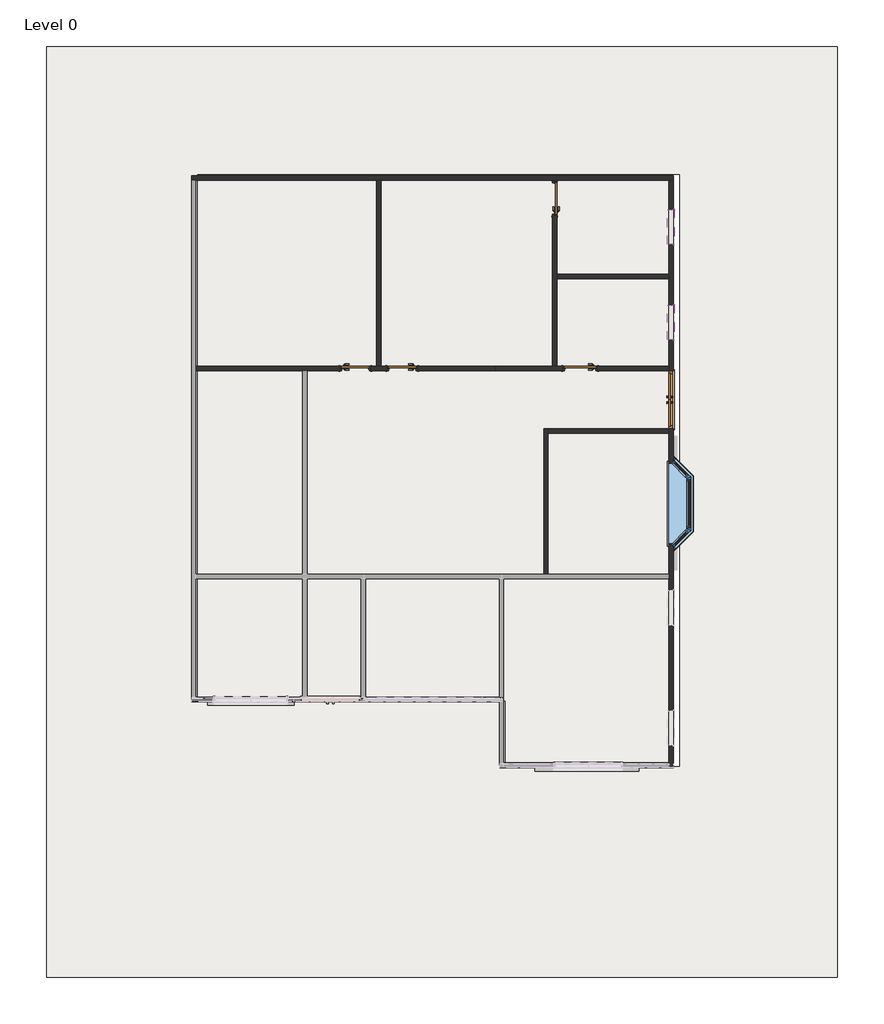
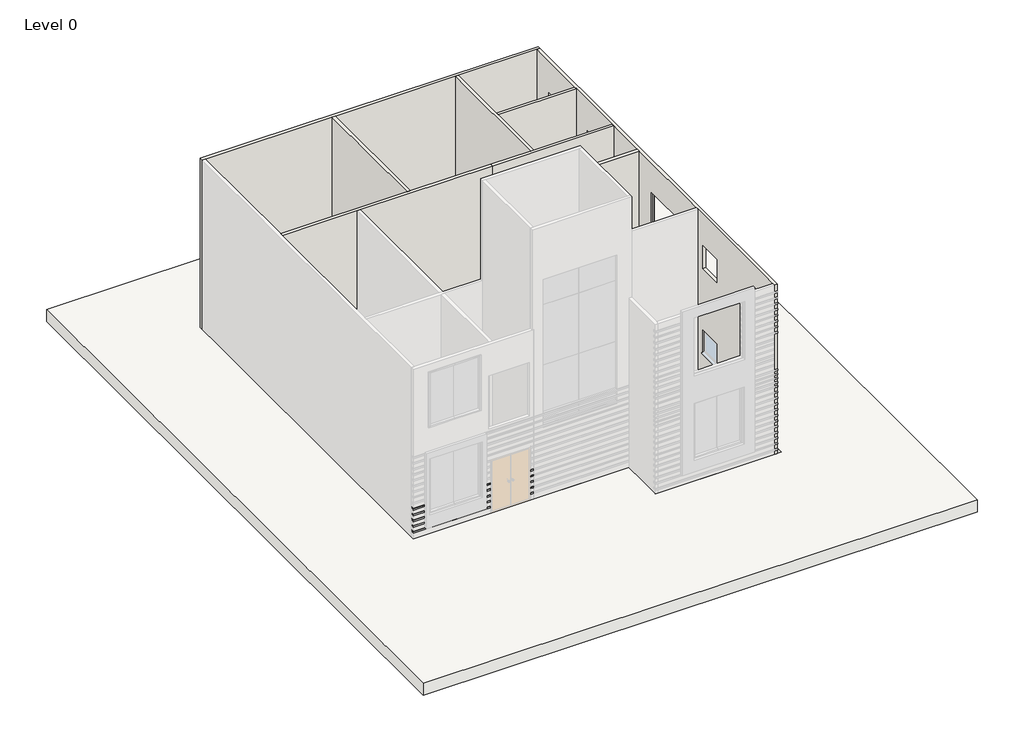
# One storey, part 4 of 5: 9 walls, 5 doors, 5 proxies, 3 windows, 2 slabs.
"""IFC4 building model written with IfcOpenShell, lengths in millimetres."""

from ifc_helpers import new_model, si_unit, frame, origin, origin_with_axes, place, context, project, spatial, polyline, outline, extrude, faceted_brep, transform, mapped, element, save
from components import doors_extdbl_flush_1510x2110mm_6aadbff8, doors_intsgl_810x2110mm_5b69c0fd, doors_intsgl_810x2110mm_5608d11f, doors_intsgl_910x2110mm_8ca64813, window_f0ba1490, windows_sgl_plain_910x910mm_53772929

model = new_model("IFC4")

# Units and contexts
model_context = context("Model", 3, world=origin())
ifc_project = project(units=[si_unit("LENGTHUNIT", "METRE", prefix="MILLI")], contexts=[model_context])

# Site, building, storey
site = spatial("IfcSite", under=ifc_project)
building = spatial("IfcBuilding", under=site)
storey = spatial("IfcBuildingStorey", under=building, Name="Level 0", Elevation=0.0)

# Proxies
placement = place(None, origin())
element("IfcBuildingElementProxy", 1, Name="Cornice", ObjectType="Cornice", at=placement, inside=storey, context=model_context, shape_type="SweptSolid", body=[
    extrude(outline(polyline([(-2780.5468048, 228.6), (-2883.0468048, 228.6), (-2883.0468048, 283.6), (-2863.0468048, 303.6), (-2780.5468048, 303.6), (-2780.5468048, 228.6)])), frame((-15018.529089, 0.0, 0.0), z_axis=(1.0, 0.0, 0.0), x_axis=(0.0, 1.0, 0.0)), (0.0, 0.0, 1.0), 107.95),
    extrude(outline(polyline([(-2780.5468048, 228.6), (-2883.0468048, 228.6), (-2883.0468048, 283.6), (-2863.0468048, 303.6), (-2780.5468048, 303.6), (-2780.5468048, 228.6)])), frame((-19412.729089, 0.0, 0.0), z_axis=(1.0, 0.0, 0.0), x_axis=(0.0, 1.0, 0.0)), (0.0, 0.0, 1.0), 2884.2),
])
element("IfcBuildingElementProxy", 2, Name="Cornice", ObjectType="Cornice", at=placement, inside=storey, context=model_context, shape_type="SweptSolid", body=[
    extrude(outline(polyline([(-2780.5468048, 457.2), (-2883.0468048, 457.2), (-2883.0468048, 512.2), (-2863.0468048, 532.2), (-2780.5468048, 532.2), (-2780.5468048, 457.2)])), frame((-15018.529089, 0.0, 0.0), z_axis=(1.0, 0.0, 0.0), x_axis=(0.0, 1.0, 0.0)), (0.0, 0.0, 1.0), 107.95),
    extrude(outline(polyline([(-2780.5468048, 457.2), (-2883.0468048, 457.2), (-2883.0468048, 512.2), (-2863.0468048, 532.2), (-2780.5468048, 532.2), (-2780.5468048, 457.2)])), frame((-19412.729089, 0.0, 0.0), z_axis=(1.0, 0.0, 0.0), x_axis=(0.0, 1.0, 0.0)), (0.0, 0.0, 1.0), 2884.2),
])
element("IfcBuildingElementProxy", 3, Name="Cornice", ObjectType="Cornice", at=placement, inside=storey, context=model_context, shape_type="SweptSolid", body=[
    extrude(outline(polyline([(-2780.5468048, 685.8), (-2883.0468048, 685.8), (-2883.0468048, 740.8), (-2863.0468048, 760.8), (-2780.5468048, 760.8), (-2780.5468048, 685.8)])), frame((-15018.529089, 0.0, 0.0), z_axis=(1.0, 0.0, 0.0), x_axis=(0.0, 1.0, 0.0)), (0.0, 0.0, 1.0), 107.95),
    extrude(outline(polyline([(-2780.5468048, 685.8), (-2883.0468048, 685.8), (-2883.0468048, 740.8), (-2863.0468048, 760.8), (-2780.5468048, 760.8), (-2780.5468048, 685.8)])), frame((-19412.729089, 0.0, 0.0), z_axis=(1.0, 0.0, 0.0), x_axis=(0.0, 1.0, 0.0)), (0.0, 0.0, 1.0), 2884.2),
])
element("IfcBuildingElementProxy", 4, Name="Cornice", ObjectType="Cornice", at=placement, inside=storey, context=model_context, shape_type="SweptSolid", body=[
    extrude(outline(polyline([(-2780.5468048, 914.4), (-2883.0468048, 914.4), (-2883.0468048, 969.4), (-2863.0468048, 989.4), (-2780.5468048, 989.4), (-2780.5468048, 914.4)])), frame((-15018.529089, 0.0, 0.0), z_axis=(1.0, 0.0, 0.0), x_axis=(0.0, 1.0, 0.0)), (0.0, 0.0, 1.0), 107.95),
    extrude(outline(polyline([(-2780.5468048, 914.4), (-2883.0468048, 914.4), (-2883.0468048, 969.4), (-2863.0468048, 989.4), (-2780.5468048, 989.4), (-2780.5468048, 914.4)])), frame((-16885.429089, 0.0, 0.0), z_axis=(1.0, 0.0, 0.0), x_axis=(0.0, 1.0, 0.0)), (0.0, 0.0, 1.0), 356.9),
    extrude(outline(polyline([(-2780.5468048, 914.4), (-2883.0468048, 914.4), (-2883.0468048, 969.4), (-2863.0468048, 989.4), (-2780.5468048, 989.4), (-2780.5468048, 914.4)])), frame((-19412.729089, 0.0, 0.0), z_axis=(1.0, 0.0, 0.0), x_axis=(0.0, 1.0, 0.0)), (0.0, 0.0, 1.0), 571.5),
])
element("IfcBuildingElementProxy", 5, Name="Cornice", ObjectType="Cornice", at=placement, inside=storey, context=model_context, shape_type="SweptSolid", body=[
    extrude(outline(polyline([(-2780.5468048, 1143.0), (-2883.0468048, 1143.0), (-2883.0468048, 1198.0), (-2863.0468048, 1218.0), (-2780.5468048, 1218.0), (-2780.5468048, 1143.0)])), frame((-15018.529089, 0.0, 0.0), z_axis=(1.0, 0.0, 0.0), x_axis=(0.0, 1.0, 0.0)), (0.0, 0.0, 1.0), 107.95),
    extrude(outline(polyline([(-2780.5468048, 1143.0), (-2883.0468048, 1143.0), (-2883.0468048, 1198.0), (-2863.0468048, 1218.0), (-2780.5468048, 1218.0), (-2780.5468048, 1143.0)])), frame((-16885.429089, 0.0, 0.0), z_axis=(1.0, 0.0, 0.0), x_axis=(0.0, 1.0, 0.0)), (0.0, 0.0, 1.0), 356.9),
    extrude(outline(polyline([(-2780.5468048, 1143.0), (-2883.0468048, 1143.0), (-2883.0468048, 1198.0), (-2863.0468048, 1218.0), (-2780.5468048, 1218.0), (-2780.5468048, 1143.0)])), frame((-19412.729089, 0.0, 0.0), z_axis=(1.0, 0.0, 0.0), x_axis=(0.0, 1.0, 0.0)), (0.0, 0.0, 1.0), 571.5),
])

# Doors
doors_extdbl_flush_1510x2110mm_shape = doors_extdbl_flush_1510x2110mm_6aadbff8(model_context)
element("IfcDoor", 6, ObjectType="Doors_ExtDbl_Flush : 1510x2110mm", at=placement, inside=storey, context=model_context, shape_type="MappedRepresentation", body=[
    mapped(doors_extdbl_flush_1510x2110mm_shape, transform((-6846.079089, 5032.7031952, 0.0), x_axis=(0.0, -1.0, 0.0), y_axis=(1.0, 0.0, 0.0), z_axis=(0.0, 0.0, 1.0))),
])
doors_intsgl_810x2110mm_shape = doors_intsgl_810x2110mm_5b69c0fd(model_context)
element("IfcDoor", 7, ObjectType="Doors_IntSgl : 810x2110mm", at=placement, inside=storey, context=model_context, shape_type="MappedRepresentation", body=[
    mapped(doors_intsgl_810x2110mm_shape, transform((-15118.729089, 5851.8531952, 0.0), x_axis=(1.0, 0.0, 0.0), y_axis=(0.0, 1.0, 0.0), z_axis=(0.0, 0.0, 1.0))),
])
doors_intsgl_810x2110mm_2_shape = doors_intsgl_810x2110mm_5608d11f(model_context)
element("IfcDoor", 8, ObjectType="Doors_IntSgl : 810x2110mm", at=placement, inside=storey, context=model_context, shape_type="MappedRepresentation", body=[
    mapped(doors_intsgl_810x2110mm_2_shape, transform((-13889.629089, 5851.8531952, 0.0), x_axis=(-1.0, 0.0, 0.0), y_axis=(0.0, -1.0, 0.0), z_axis=(0.0, 0.0, 1.0))),
])
doors_intsgl_910x2110mm_shape = doors_intsgl_910x2110mm_8ca64813(model_context)
element("IfcDoor", 9, ObjectType="Doors_IntSgl : 910x2110mm", at=placement, inside=storey, context=model_context, shape_type="MappedRepresentation", body=[
    mapped(doors_intsgl_910x2110mm_shape, transform((-9894.079089, 10305.4031952, 0.0), x_axis=(0.0, 1.0, 0.0), y_axis=(-1.0, 0.0, 0.0), z_axis=(0.0, 0.0, 1.0))),
])
element("IfcDoor", 10, ObjectType="Doors_IntSgl : 910x2110mm", at=placement, inside=storey, context=model_context, shape_type="MappedRepresentation", body=[
    mapped(doors_intsgl_910x2110mm_shape, transform((-9229.529089, 5851.8531952, 0.0), x_axis=(-1.0, 0.0, 0.0), y_axis=(0.0, -1.0, 0.0), z_axis=(0.0, 0.0, 1.0))),
])

# Slabs
element("IfcSlab", 11, ObjectType="Floor-Grnd-Susp_65Scr-80Ins-100Blk-75PC", at=placement, inside=storey, context=model_context, shape_type="SweptSolid", body=[
    extrude(outline(polyline([(-19412.729089, 10900.1031952), (-6788.929089, 10900.1031952), (-6788.929089, -4593.8968048), (-11348.229089, -4593.8968048), (-11348.229089, -2873.0468048), (-19412.729089, -2873.0468048), (-19412.729089, 10900.1031952)])), frame((0.0, 0.0, -470.0), z_axis=(0.0, 0.0, 1.0), x_axis=(1.0, 0.0, 0.0)), (0.0, 0.0, 1.0), 470.0),
])
element("IfcSlab", 12, ObjectType="Floor-Grnd-Susp_65Scr-80Ins-100Blk-75PC", at=placement, inside=storey, context=model_context, shape_type="SweptSolid", body=[
    extrude(outline(polyline([(-2486.7820212, 14284.0681415), (-2486.7820212, -10099.9318585), (-23213.1820212, -10099.9318585), (-23213.1820212, 14284.0681415), (-2486.7820212, 14284.0681415)]), holes=[polyline([(-19254.3177331, 10923.6963759), (-19254.3177331, -2849.4536241), (-11189.8177331, -2849.4536241), (-11189.8177331, -4570.3036241), (-6630.5177331, -4570.3036241), (-6630.5177331, 10923.6963759), (-19254.3177331, 10923.6963759)])]), frame((0.0, 0.0, -470.0), z_axis=(0.0, 0.0, 1.0), x_axis=(1.0, 0.0, 0.0)), (0.0, 0.0, 1.0), 470.0),
])

# Walls
element("IfcWall", 13, ObjectType="basic wall", at=placement, inside=storey, context=model_context, shape_type="Brep", body=[
    faceted_brep([(-19412.729089, 10785.8031952, 0.0), (-19298.429089, 10785.8031952, 0.0), (-14561.329089, 10785.8031952, 0.0), (-14447.029089, 10785.8031952, 0.0), (-9951.229089, 10785.8031952, 0.0), (-9836.929089, 10785.8031952, 0.0), (-6903.229089, 10785.8031952, 0.0), (-6788.929089, 10785.8031952, 0.0), (-6788.929089, 10785.8031952, 6705.6), (-6903.229089, 10785.8031952, 6705.6), (-9836.929089, 10785.8031952, 6705.6), (-9951.229089, 10785.8031952, 6705.6), (-14447.029089, 10785.8031952, 6705.6), (-14561.329089, 10785.8031952, 6705.6), (-19298.429089, 10785.8031952, 6705.6), (-19412.729089, 10785.8031952, 6705.6), (-19412.729089, 10900.1031952, 0.0), (-19412.729089, 10900.1031952, 6705.6), (-6788.929089, 10900.1031952, 6705.6), (-6788.929089, 10900.1031952, 0.0)], [[[0, 1, 2, 3, 4, 5, 6, 7, 8, 9, 10, 11, 12, 13, 14, 15]], [[16, 17, 18, 19]], [[7, 6, 5, 4, 3, 2, 1, 0, 16, 19]], [[15, 14, 13, 12, 11, 10, 9, 8, 18, 17]], [[8, 7, 19, 18]], [[0, 15, 17, 16]]]),
])
element("IfcWall", 14, ObjectType="basic wall", at=placement, inside=storey, context=model_context, shape_type="Brep", body=[
    faceted_brep([(-10065.529089, 460.7031952, 0.0), (-10065.529089, 4156.4031952, 0.0), (-10065.529089, 4270.7031952, 0.0), (-10065.529089, 4270.7031952, 6705.6), (-10065.529089, 4156.4031952, 6705.6), (-10065.529089, 460.7031952, 6705.6), (-10179.829089, 460.7031952, 0.0), (-10179.829089, 460.7031952, 6705.6), (-10179.829089, 4270.7031952, 6705.6), (-10179.829089, 4270.7031952, 0.0)], [[[0, 1, 2, 3, 4, 5]], [[6, 7, 8, 9]], [[2, 1, 0, 6, 9]], [[5, 4, 3, 8, 7]], [[0, 5, 7, 6]], [[3, 2, 9, 8]]]),
])
element("IfcWall", 15, ObjectType="basic wall", at=placement, inside=storey, context=model_context, shape_type="SweptSolid", body=[
    extrude(outline(polyline([(-6903.229089, 4156.4031952), (-10065.529089, 4156.4031952), (-10065.529089, 4270.7031952), (-6903.229089, 4270.7031952), (-6903.229089, 4156.4031952)])), origin_with_axes(), (0.0, 0.0, 1.0), 6705.6),
])
element("IfcWall", 16, ObjectType="basic wall", at=placement, inside=storey, context=model_context, shape_type="Brep", body=[
    faceted_brep([(-11449.829089, 5909.0031952, 0.0), (-11449.829089, 5909.0031952, 6705.6), (-9951.229089, 5909.0031952, 6705.6), (-9836.929089, 5909.0031952, 6705.6), (-6903.229089, 5909.0031952, 6705.6), (-6903.229089, 5909.0031952, 0.0), (-8774.529089, 5909.0031952, 0.0), (-8774.529089, 5909.0031952, 2110.0), (-9684.529089, 5909.0031952, 2110.0), (-9684.529089, 5909.0031952, 0.0), (-9836.929089, 5909.0031952, 0.0), (-9951.229089, 5909.0031952, 0.0), (-11449.829089, 5794.7031952, 6705.6), (-11449.829089, 5794.7031952, 0.0), (-9684.529089, 5794.7031952, 0.0), (-9684.529089, 5794.7031952, 2110.0), (-8774.529089, 5794.7031952, 2110.0), (-8774.529089, 5794.7031952, 0.0), (-6903.229089, 5794.7031952, 0.0), (-6903.229089, 5794.7031952, 6705.6)], [[[0, 1, 2, 3, 4, 5, 6, 7, 8, 9, 10, 11]], [[12, 13, 14, 15, 16, 17, 18, 19]], [[5, 18, 17, 6]], [[13, 0, 11, 10, 9, 14]], [[1, 0, 13, 12]], [[4, 3, 2, 1, 12, 19]], [[5, 4, 19, 18]], [[8, 15, 14, 9]], [[15, 8, 7, 16]], [[16, 7, 6, 17]]]),
])
element("IfcWall", 17, ObjectType="basic wall", at=placement, inside=storey, context=model_context, shape_type="SweptSolid", body=[
    extrude(outline(polyline([(-9836.929089, 8322.0031952), (-6903.229089, 8322.0031952), (-6903.229089, 8207.7031952), (-9836.929089, 8207.7031952), (-9836.929089, 8322.0031952)])), origin_with_axes(), (0.0, 0.0, 1.0), 6705.6),
])
element("IfcWall", 18, ObjectType="basic wall", at=placement, inside=storey, context=model_context, shape_type="Brep", body=[
    faceted_brep([(-9836.929089, 10785.8031952, 6705.6), (-9836.929089, 8322.0031952, 6705.6), (-9836.929089, 8207.7031952, 6705.6), (-9836.929089, 5909.0031952, 6705.6), (-9836.929089, 5909.0031952, 0.0), (-9836.929089, 8207.7031952, 0.0), (-9836.929089, 8322.0031952, 0.0), (-9836.929089, 9850.4031952, 0.0), (-9836.929089, 9850.4031952, 2110.0), (-9836.929089, 10760.4031952, 2110.0), (-9836.929089, 10760.4031952, 0.0), (-9836.929089, 10785.8031952, 0.0), (-9951.229089, 5909.0031952, 6705.6), (-9951.229089, 10785.8031952, 6705.6), (-9951.229089, 10785.8031952, 0.0), (-9951.229089, 10760.4031952, 0.0), (-9951.229089, 10760.4031952, 2110.0), (-9951.229089, 9850.4031952, 2110.0), (-9951.229089, 9850.4031952, 0.0), (-9951.229089, 5909.0031952, 0.0)], [[[0, 1, 2, 3, 4, 5, 6, 7, 8, 9, 10, 11]], [[12, 13, 14, 15, 16, 17, 18, 19]], [[14, 11, 10, 15]], [[4, 19, 18, 7, 6, 5]], [[3, 2, 1, 0, 13, 12]], [[0, 11, 14, 13]], [[4, 3, 12, 19]], [[9, 16, 15, 10]], [[16, 9, 8, 17]], [[17, 8, 7, 18]]]),
])
element("IfcWall", 19, ObjectType="basic wall", at=placement, inside=storey, context=model_context, shape_type="SweptSolid", body=[
    extrude(outline(polyline([(-14561.329089, 5909.0031952), (-14561.329089, 10785.8031952), (-14447.029089, 10785.8031952), (-14447.029089, 5909.0031952), (-14561.329089, 5909.0031952)])), origin_with_axes(), (0.0, 0.0, 1.0), 6705.6),
])
element("IfcWall", 20, ObjectType="basic wall", at=placement, inside=storey, context=model_context, shape_type="Brep", body=[
    faceted_brep([(-19298.429089, 5909.0031952, 6705.6), (-14561.329089, 5909.0031952, 6705.6), (-14447.029089, 5909.0031952, 6705.6), (-11449.829089, 5909.0031952, 6705.6), (-11449.829089, 5909.0031952, 0.0), (-13484.629089, 5909.0031952, 0.0), (-13484.629089, 5909.0031952, 2110.0), (-14294.629089, 5909.0031952, 2110.0), (-14294.629089, 5909.0031952, 0.0), (-14447.029089, 5909.0031952, 0.0), (-14561.329089, 5909.0031952, 0.0), (-14713.729089, 5909.0031952, 0.0), (-14713.729089, 5909.0031952, 2110.0), (-15523.729089, 5909.0031952, 2110.0), (-15523.729089, 5909.0031952, 0.0), (-19298.429089, 5909.0031952, 0.0), (-11449.829089, 5794.7031952, 6705.6), (-16390.129089, 5794.7031952, 6705.6), (-16504.429089, 5794.7031952, 6705.6), (-19298.429089, 5794.7031952, 6705.6), (-19298.429089, 5794.7031952, 0.0), (-16504.429089, 5794.7031952, 0.0), (-16390.129089, 5794.7031952, 0.0), (-15523.729089, 5794.7031952, 0.0), (-15523.729089, 5794.7031952, 2110.0), (-14713.729089, 5794.7031952, 2110.0), (-14713.729089, 5794.7031952, 0.0), (-14294.629089, 5794.7031952, 0.0), (-14294.629089, 5794.7031952, 2110.0), (-13484.629089, 5794.7031952, 2110.0), (-13484.629089, 5794.7031952, 0.0), (-11449.829089, 5794.7031952, 0.0)], [[[0, 1, 2, 3, 4, 5, 6, 7, 8, 9, 10, 11, 12, 13, 14, 15]], [[16, 17, 18, 19, 20, 21, 22, 23, 24, 25, 26, 27, 28, 29, 30, 31]], [[20, 15, 14, 23, 22, 21]], [[4, 31, 30, 5]], [[26, 11, 10, 9, 8, 27]], [[3, 2, 1, 0, 19, 18, 17, 16]], [[4, 3, 16, 31]], [[0, 15, 20, 19]], [[25, 12, 11, 26]], [[12, 25, 24, 13]], [[13, 24, 23, 14]], [[7, 28, 27, 8]], [[28, 7, 6, 29]], [[29, 6, 5, 30]]]),
])
element("IfcWall", 21, ObjectType="basic wall 8", at=placement, inside=storey, context=model_context, shape_type="Brep", body=[
    faceted_brep([(-6903.229089, -4593.8968048, 6705.6), (-6903.229089, -4479.5968048, 6705.6), (-6903.229089, 346.4031952, 6705.6), (-6903.229089, 460.7031952, 6705.6), (-6903.229089, 4156.4031952, 6705.6), (-6903.229089, 4270.7031952, 6705.6), (-6903.229089, 5794.7031952, 6705.6), (-6903.229089, 5909.0031952, 6705.6), (-6903.229089, 8207.7031952, 6705.6), (-6903.229089, 8322.0031952, 6705.6), (-6903.229089, 10785.8031952, 6705.6), (-6903.229089, 10785.8031952, 0.0), (-6903.229089, 8322.0031952, 0.0), (-6903.229089, 8207.7031952, 0.0), (-6903.229089, 5909.0031952, 0.0), (-6903.229089, 5794.7031952, 0.0), (-6903.229089, 5787.7031952, 0.0), (-6903.229089, 5787.7031952, 2110.0), (-6903.229089, 4277.7031952, 2110.0), (-6903.229089, 4277.7031952, 0.0), (-6903.229089, 4270.7031952, 0.0), (-6903.229089, 4156.4031952, 0.0), (-6903.229089, 460.7031952, 0.0), (-6903.229089, 346.4031952, 0.0), (-6903.229089, -4479.5968048, 0.0), (-6903.229089, -4593.8968048, 0.0), (-6903.229089, -4593.8968048, 152.4), (-6903.229089, -4501.3968048, 152.4), (-6903.229089, -4501.3968048, 227.4), (-6903.229089, -4583.8968048, 227.4), (-6903.229089, -4593.8968048, 217.4), (-6903.229089, -4593.8968048, 381.0), (-6903.229089, -4501.3968048, 381.0), (-6903.229089, -4501.3968048, 456.0), (-6903.229089, -4583.8968048, 456.0), (-6903.229089, -4593.8968048, 446.0), (-6903.229089, -4593.8968048, 609.6), (-6903.229089, -4501.3968048, 609.6), (-6903.229089, -4501.3968048, 684.6), (-6903.229089, -4583.8968048, 684.6), (-6903.229089, -4593.8968048, 674.6), (-6903.229089, -4593.8968048, 830.4106439), (-6903.229089, -4501.3968048, 830.4106439), (-6903.229089, -4501.3968048, 905.4106439), (-6903.229089, -4583.8968048, 905.4106439), (-6903.229089, -4593.8968048, 895.4106439), (-6903.229089, -4593.8968048, 1059.0106439), (-6903.229089, -4501.3968048, 1059.0106439), (-6903.229089, -4501.3968048, 1134.0106439), (-6903.229089, -4583.8968048, 1134.0106439), (-6903.229089, -4593.8968048, 1124.0106439), (-6903.229089, -4593.8968048, 1279.8212878), (-6903.229089, -4501.3968048, 1279.8212878), (-6903.229089, -4501.3968048, 1354.8212878), (-6903.229089, -4583.8968048, 1354.8212878), (-6903.229089, -4593.8968048, 1344.8212878), (-6903.229089, -4593.8968048, 1500.6319317), (-6903.229089, -4501.3968048, 1500.6319317), (-6903.229089, -4501.3968048, 1575.6319317), (-6903.229089, -4583.8968048, 1575.6319317), (-6903.229089, -4593.8968048, 1565.6319317), (-6903.229089, -4593.8968048, 1729.2319317), (-6903.229089, -4501.3968048, 1729.2319317), (-6903.229089, -4501.3968048, 1804.2319317), (-6903.229089, -4583.8968048, 1804.2319317), (-6903.229089, -4593.8968048, 1794.2319317), (-6903.229089, -4593.8968048, 1957.8319317), (-6903.229089, -4501.3968048, 1957.8319317), (-6903.229089, -4501.3968048, 2032.8319317), (-6903.229089, -4583.8968048, 2032.8319317), (-6903.229089, -4593.8968048, 2022.8319317), (-6903.229089, -4593.8968048, 2186.4319317), (-6903.229089, -4501.3968048, 2186.4319317), (-6903.229089, -4501.3968048, 2261.4319317), (-6903.229089, -4583.8968048, 2261.4319317), (-6903.229089, -4593.8968048, 2251.4319317), (-6903.229089, -4593.8968048, 2415.0319317), (-6903.229089, -4501.3968048, 2415.0319317), (-6903.229089, -4501.3968048, 2490.0319317), (-6903.229089, -4583.8968048, 2490.0319317), (-6903.229089, -4593.8968048, 2480.0319317), (-6903.229089, -4593.8968048, 2643.6319317), (-6903.229089, -4501.3968048, 2643.6319317), (-6903.229089, -4501.3968048, 2718.6319317), (-6903.229089, -4583.8968048, 2718.6319317), (-6903.229089, -4593.8968048, 2708.6319317), (-6903.229089, -4593.8968048, 2805.2765418), (-6903.229089, -4501.3968048, 2805.2765418), (-6903.229089, -4501.3968048, 2880.2765418), (-6903.229089, -4583.8968048, 2880.2765418), (-6903.229089, -4593.8968048, 2870.2765418), (-6903.229089, -4593.8968048, 2966.921152), (-6903.229089, -4501.3968048, 2966.921152), (-6903.229089, -4501.3968048, 3041.921152), (-6903.229089, -4583.8968048, 3041.921152), (-6903.229089, -4593.8968048, 3031.921152), (-6903.229089, -4593.8968048, 3128.5657622), (-6903.229089, -4501.3968048, 3128.5657622), (-6903.229089, -4501.3968048, 3203.5657622), (-6903.229089, -4583.8968048, 3203.5657622), (-6903.229089, -4593.8968048, 3193.5657622), (-6903.229089, -4593.8968048, 3290.2103724), (-6903.229089, -4501.3968048, 3290.2103724), (-6903.229089, -4501.3968048, 3365.2103724), (-6903.229089, -4583.8968048, 3365.2103724), (-6903.229089, -4593.8968048, 3355.2103724), (-6903.229089, -4593.8968048, 3518.8103724), (-6903.229089, -4593.8968048, 3583.8103724), (-6903.229089, -4593.8968048, 3747.4103724), (-6903.229089, -4593.8968048, 3812.4103724), (-6903.229089, -4593.8968048, 3909.0549826), (-6903.229089, -4593.8968048, 3974.0549826), (-6903.229089, -4593.8968048, 4137.6549826), (-6903.229089, -4593.8968048, 4202.6549826), (-6903.229089, -4593.8968048, 4358.4656265), (-6903.229089, -4593.8968048, 4423.4656265), (-6903.229089, -4593.8968048, 4545.5846362), (-6903.229089, -4593.8968048, 4610.5846362), (-6903.229089, -4593.8968048, 4774.1846362), (-6903.229089, -4501.3968048, 4774.1846362), (-6903.229089, -4501.3968048, 4849.1846362), (-6903.229089, -4583.8968048, 4849.1846362), (-6903.229089, -4593.8968048, 4839.1846362), (-6903.229089, -4593.8968048, 5002.7846362), (-6903.229089, -4501.3968048, 5002.7846362), (-6903.229089, -4501.3968048, 5077.7846362), (-6903.229089, -4583.8968048, 5077.7846362), (-6903.229089, -4593.8968048, 5067.7846362), (-6903.229089, -4593.8968048, 5231.3846362), (-6903.229089, -4501.3968048, 5231.3846362), (-6903.229089, -4501.3968048, 5306.3846362), (-6903.229089, -4583.8968048, 5306.3846362), (-6903.229089, -4593.8968048, 5296.3846362), (-6903.229089, -4593.8968048, 5459.9846362), (-6903.229089, -4501.3968048, 5459.9846362), (-6903.229089, -4501.3968048, 5534.9846362), (-6903.229089, -4583.8968048, 5534.9846362), (-6903.229089, -4593.8968048, 5524.9846362), (-6903.229089, -4593.8968048, 5688.5846362), (-6903.229089, -4501.3968048, 5688.5846362), (-6903.229089, -4501.3968048, 5763.5846362), (-6903.229089, -4583.8968048, 5763.5846362), (-6903.229089, -4593.8968048, 5753.5846362), (-6903.229089, -4593.8968048, 5917.1846362), (-6903.229089, -4501.3968048, 5917.1846362), (-6903.229089, -4501.3968048, 5992.1846362), (-6903.229089, -4583.8968048, 5992.1846362), (-6903.229089, -4593.8968048, 5982.1846362), (-6903.229089, -4593.8968048, 6145.7846362), (-6903.229089, -4501.3968048, 6145.7846362), (-6903.229089, -4501.3968048, 6220.7846362), (-6903.229089, -4583.8968048, 6220.7846362), (-6903.229089, -4593.8968048, 6210.7846362), (-6903.229089, -4593.8968048, 6374.3846362), (-6903.229089, -4501.3968048, 6374.3846362), (-6903.229089, -4501.3968048, 6449.3846362), (-6903.229089, -4583.8968048, 6449.3846362), (-6903.229089, -4593.8968048, 6439.3846362), (-6903.229089, -868.3968048, 2110.0), (-6903.229089, -868.3968048, 1200.0), (-6903.229089, 41.6031952, 1200.0), (-6903.229089, 41.6031952, 2110.0), (-6903.229089, -4022.3968048, 2110.0), (-6903.229089, -4022.3968048, 1200.0), (-6903.229089, -3112.3968048, 1200.0), (-6903.229089, -3112.3968048, 2110.0), (-6903.229089, 6603.3531952, 2110.0), (-6903.229089, 6603.3531952, 1200.0), (-6903.229089, 7513.3531952, 1200.0), (-6903.229089, 7513.3531952, 2110.0), (-6903.229089, 9098.9031952, 2110.0), (-6903.229089, 9098.9031952, 1200.0), (-6903.229089, 10008.9031952, 1200.0), (-6903.229089, 10008.9031952, 2110.0), (-6903.229089, 5787.7031952, 3352.8), (-6903.229089, 5787.7031952, 5462.8), (-6903.229089, 4277.7031952, 5462.8), (-6903.229089, 4277.7031952, 3352.8), (-6903.229089, 3375.3531952, 5537.2), (-6903.229089, 1241.7531952, 5537.2), (-6903.229089, 1241.7531952, 3962.4), (-6903.229089, 3375.3531952, 3962.4), (-6903.229089, 9098.9031952, 5462.8), (-6903.229089, 9098.9031952, 4552.8), (-6903.229089, 10008.9031952, 4552.8), (-6903.229089, 10008.9031952, 5462.8), (-6903.229089, 6603.3531952, 5462.8), (-6903.229089, 6603.3531952, 4552.8), (-6903.229089, 7513.3531952, 4552.8), (-6903.229089, 7513.3531952, 5462.8), (-6903.229089, -4022.3968048, 5462.8), (-6903.229089, -4022.3968048, 4552.8), (-6903.229089, -3112.3968048, 4552.8), (-6903.229089, -3112.3968048, 5462.8), (-6903.229089, -868.3968048, 5462.8), (-6903.229089, -868.3968048, 4552.8), (-6903.229089, 41.6031952, 4552.8), (-6903.229089, 41.6031952, 5462.8), (-6903.229089, 3375.3531952, 2184.4), (-6903.229089, 1241.7531952, 2184.4), (-6903.229089, 1241.7531952, 609.6), (-6903.229089, 3375.3531952, 609.6), (-6788.929089, 10785.8031952, 6705.6), (-6788.929089, -4593.8968048, 6705.6), (-6788.929089, -4593.8968048, 6439.3846362), (-6788.929089, -4583.8968048, 6449.3846362), (-6788.929089, -4501.3968048, 6449.3846362), (-6788.929089, -4501.3968048, 6374.3846362), (-6788.929089, -4593.8968048, 6374.3846362), (-6788.929089, -4593.8968048, 6210.7846362), (-6788.929089, -4583.8968048, 6220.7846362), (-6788.929089, -4501.3968048, 6220.7846362), (-6788.929089, -4501.3968048, 6145.7846362), (-6788.929089, -4593.8968048, 6145.7846362), (-6788.929089, -4593.8968048, 5982.1846362), (-6788.929089, -4583.8968048, 5992.1846362), (-6788.929089, -4501.3968048, 5992.1846362), (-6788.929089, -4501.3968048, 5917.1846362), (-6788.929089, -4593.8968048, 5917.1846362), (-6788.929089, -4593.8968048, 5753.5846362), (-6788.929089, -4583.8968048, 5763.5846362), (-6788.929089, -4501.3968048, 5763.5846362), (-6788.929089, -4501.3968048, 5688.5846362), (-6788.929089, -4593.8968048, 5688.5846362), (-6788.929089, -4593.8968048, 5524.9846362), (-6788.929089, -4583.8968048, 5534.9846362), (-6788.929089, -4501.3968048, 5534.9846362), (-6788.929089, -4501.3968048, 5459.9846362), (-6788.929089, -4593.8968048, 5459.9846362), (-6788.929089, -4593.8968048, 5296.3846362), (-6788.929089, -4583.8968048, 5306.3846362), (-6788.929089, -4501.3968048, 5306.3846362), (-6788.929089, -4501.3968048, 5231.3846362), (-6788.929089, -4593.8968048, 5231.3846362), (-6788.929089, -4593.8968048, 5067.7846362), (-6788.929089, -4583.8968048, 5077.7846362), (-6788.929089, -4501.3968048, 5077.7846362), (-6788.929089, -4501.3968048, 5002.7846362), (-6788.929089, -4593.8968048, 5002.7846362), (-6788.929089, -4593.8968048, 4839.1846362), (-6788.929089, -4583.8968048, 4849.1846362), (-6788.929089, -4501.3968048, 4849.1846362), (-6788.929089, -4501.3968048, 4774.1846362), (-6788.929089, -4593.8968048, 4774.1846362), (-6788.929089, -4593.8968048, 4572.0), (-6788.929089, -4593.8968048, 3355.2103724), (-6788.929089, -4583.8968048, 3365.2103724), (-6788.929089, -4501.3968048, 3365.2103724), (-6788.929089, -4501.3968048, 3290.2103724), (-6788.929089, -4593.8968048, 3290.2103724), (-6788.929089, -4593.8968048, 3193.5657622), (-6788.929089, -4583.8968048, 3203.5657622), (-6788.929089, -4501.3968048, 3203.5657622), (-6788.929089, -4501.3968048, 3128.5657622), (-6788.929089, -4593.8968048, 3128.5657622), (-6788.929089, -4593.8968048, 3031.921152), (-6788.929089, -4583.8968048, 3041.921152), (-6788.929089, -4501.3968048, 3041.921152), (-6788.929089, -4501.3968048, 2966.921152), (-6788.929089, -4593.8968048, 2966.921152), (-6788.929089, -4593.8968048, 2870.2765418), (-6788.929089, -4583.8968048, 2880.2765418), (-6788.929089, -4501.3968048, 2880.2765418), (-6788.929089, -4501.3968048, 2805.2765418), (-6788.929089, -4593.8968048, 2805.2765418), (-6788.929089, -4593.8968048, 2708.6319317), (-6788.929089, -4583.8968048, 2718.6319317), (-6788.929089, -4501.3968048, 2718.6319317), (-6788.929089, -4501.3968048, 2643.6319317), (-6788.929089, -4593.8968048, 2643.6319317), (-6788.929089, -4593.8968048, 2480.0319317), (-6788.929089, -4583.8968048, 2490.0319317), (-6788.929089, -4501.3968048, 2490.0319317), (-6788.929089, -4501.3968048, 2415.0319317), (-6788.929089, -4593.8968048, 2415.0319317), (-6788.929089, -4593.8968048, 2251.4319317), (-6788.929089, -4583.8968048, 2261.4319317), (-6788.929089, -4501.3968048, 2261.4319317), (-6788.929089, -4501.3968048, 2186.4319317), (-6788.929089, -4593.8968048, 2186.4319317), (-6788.929089, -4593.8968048, 2022.8319317), (-6788.929089, -4583.8968048, 2032.8319317), (-6788.929089, -4501.3968048, 2032.8319317), (-6788.929089, -4501.3968048, 1957.8319317), (-6788.929089, -4593.8968048, 1957.8319317), (-6788.929089, -4593.8968048, 1794.2319317), (-6788.929089, -4583.8968048, 1804.2319317), (-6788.929089, -4501.3968048, 1804.2319317), (-6788.929089, -4501.3968048, 1729.2319317), (-6788.929089, -4593.8968048, 1729.2319317), (-6788.929089, -4593.8968048, 1565.6319317), (-6788.929089, -4583.8968048, 1575.6319317), (-6788.929089, -4501.3968048, 1575.6319317), (-6788.929089, -4501.3968048, 1500.6319317), (-6788.929089, -4593.8968048, 1500.6319317), (-6788.929089, -4593.8968048, 1344.8212878), (-6788.929089, -4583.8968048, 1354.8212878), (-6788.929089, -4501.3968048, 1354.8212878), (-6788.929089, -4501.3968048, 1279.8212878), (-6788.929089, -4593.8968048, 1279.8212878), (-6788.929089, -4593.8968048, 1124.0106439), (-6788.929089, -4583.8968048, 1134.0106439), (-6788.929089, -4501.3968048, 1134.0106439), (-6788.929089, -4501.3968048, 1059.0106439), (-6788.929089, -4593.8968048, 1059.0106439), (-6788.929089, -4593.8968048, 895.4106439), (-6788.929089, -4583.8968048, 905.4106439), (-6788.929089, -4501.3968048, 905.4106439), (-6788.929089, -4501.3968048, 830.4106439), (-6788.929089, -4593.8968048, 830.4106439), (-6788.929089, -4593.8968048, 674.6), (-6788.929089, -4583.8968048, 684.6), (-6788.929089, -4501.3968048, 684.6), (-6788.929089, -4501.3968048, 609.6), (-6788.929089, -4593.8968048, 609.6), (-6788.929089, -4593.8968048, 446.0), (-6788.929089, -4583.8968048, 456.0), (-6788.929089, -4501.3968048, 456.0), (-6788.929089, -4501.3968048, 381.0), (-6788.929089, -4593.8968048, 381.0), (-6788.929089, -4593.8968048, 217.4), (-6788.929089, -4583.8968048, 227.4), (-6788.929089, -4501.3968048, 227.4), (-6788.929089, -4501.3968048, 152.4), (-6788.929089, -4593.8968048, 152.4), (-6788.929089, -4593.8968048, 0.0), (-6788.929089, 4277.7031952, 0.0), (-6788.929089, 4277.7031952, 2110.0), (-6788.929089, 5787.7031952, 2110.0), (-6788.929089, 5787.7031952, 0.0), (-6788.929089, 10785.8031952, 0.0), (-6788.929089, -868.3968048, 1200.0), (-6788.929089, -868.3968048, 2110.0), (-6788.929089, 41.6031952, 2110.0), (-6788.929089, 41.6031952, 1200.0), (-6788.929089, -4022.3968048, 1200.0), (-6788.929089, -4022.3968048, 2110.0), (-6788.929089, -3112.3968048, 2110.0), (-6788.929089, -3112.3968048, 1200.0), (-6788.929089, 6603.3531952, 1200.0), (-6788.929089, 6603.3531952, 2110.0), (-6788.929089, 7513.3531952, 2110.0), (-6788.929089, 7513.3531952, 1200.0), (-6788.929089, 9098.9031952, 1200.0), (-6788.929089, 9098.9031952, 2110.0), (-6788.929089, 10008.9031952, 2110.0), (-6788.929089, 10008.9031952, 1200.0), (-6788.929089, 5787.7031952, 5462.8), (-6788.929089, 5787.7031952, 3352.8), (-6788.929089, 4277.7031952, 3352.8), (-6788.929089, 4277.7031952, 5462.8), (-6788.929089, 1192.3617866, 5537.2), (-6788.929089, 3424.7446039, 5537.2), (-6788.929089, 3424.7446039, 3962.4), (-6788.929089, 1192.3617866, 3962.4), (-6788.929089, 9098.9031952, 4552.8), (-6788.929089, 9098.9031952, 5462.8), (-6788.929089, 10008.9031952, 5462.8), (-6788.929089, 10008.9031952, 4552.8), (-6788.929089, 6603.3531952, 4552.8), (-6788.929089, 6603.3531952, 5462.8), (-6788.929089, 7513.3531952, 5462.8), (-6788.929089, 7513.3531952, 4552.8), (-6788.929089, -4022.3968048, 4552.8), (-6788.929089, -4022.3968048, 5462.8), (-6788.929089, -3112.3968048, 5462.8), (-6788.929089, -3112.3968048, 4552.8), (-6788.929089, -868.3968048, 4552.8), (-6788.929089, -868.3968048, 5462.8), (-6788.929089, 41.6031952, 5462.8), (-6788.929089, 41.6031952, 4552.8), (-6788.929089, 1192.3617866, 2184.4), (-6788.929089, 3424.7446039, 2184.4), (-6788.929089, 3424.7446039, 609.6), (-6788.929089, 1192.3617866, 609.6), (-6838.3204977, 3375.3531952, 5537.2), (-6838.3204977, 1241.7531952, 5537.2), (-6838.3204977, 3375.3531952, 3962.4), (-6838.3204977, 1241.7531952, 3962.4), (-6838.3204977, 3375.3531952, 2184.4), (-6838.3204977, 1241.7531952, 2184.4), (-6838.3204977, 3375.3531952, 609.6), (-6838.3204977, 1241.7531952, 609.6)], [[[0, 1, 2, 3, 4, 5, 6, 7, 8, 9, 10, 11, 12, 13, 14, 15, 16, 17, 18, 19, 20, 21, 22, 23, 24, 25, 26, 27, 28, 29, 30, 31, 32, 33, 34, 35, 36, 37, 38, 39, 40, 41, 42, 43, 44, 45, 46, 47, 48, 49, 50, 51, 52, 53, 54, 55, 56, 57, 58, 59, 60, 61, 62, 63, 64, 65, 66, 67, 68, 69, 70, 71, 72, 73, 74, 75, 76, 77, 78, 79, 80, 81, 82, 83, 84, 85, 86, 87, 88, 89, 90, 91, 92, 93, 94, 95, 96, 97, 98, 99, 100, 101, 102, 103, 104, 105, 106, 107, 108, 109, 110, 111, 112, 113, 114, 115, 116, 117, 118, 119, 120, 121, 122, 123, 124, 125, 126, 127, 128, 129, 130, 131, 132, 133, 134, 135, 136, 137, 138, 139, 140, 141, 142, 143, 144, 145, 146, 147, 148, 149, 150, 151, 152, 153, 154, 155, 156, 157], [158, 159, 160, 161], [162, 163, 164, 165], [166, 167, 168, 169], [170, 171, 172, 173], [174, 175, 176, 177], [178, 179, 180, 181], [182, 183, 184, 185], [186, 187, 188, 189], [190, 191, 192, 193], [194, 195, 196, 197], [198, 199, 200, 201]], [[202, 203, 204, 205, 206, 207, 208, 209, 210, 211, 212, 213, 214, 215, 216, 217, 218, 219, 220, 221, 222, 223, 224, 225, 226, 227, 228, 229, 230, 231, 232, 233, 234, 235, 236, 237, 238, 239, 240, 241, 242, 243, 244, 245, 246, 247, 248, 249, 250, 251, 252, 253, 254, 255, 256, 257, 258, 259, 260, 261, 262, 263, 264, 265, 266, 267, 268, 269, 270, 271, 272, 273, 274, 275, 276, 277, 278, 279, 280, 281, 282, 283, 284, 285, 286, 287, 288, 289, 290, 291, 292, 293, 294, 295, 296, 297, 298, 299, 300, 301, 302, 303, 304, 305, 306, 307, 308, 309, 310, 311, 312, 313, 314, 315, 316, 317, 318, 319, 320, 321, 322, 323, 324, 325, 326, 327, 328, 329, 330], [331, 332, 333, 334], [335, 336, 337, 338], [339, 340, 341, 342], [343, 344, 345, 346], [347, 348, 349, 350], [351, 352, 353, 354], [355, 356, 357, 358], [359, 360, 361, 362], [363, 364, 365, 366], [367, 368, 369, 370], [371, 372, 373, 374]], [[11, 330, 329, 16, 15, 14, 13, 12]], [[325, 25, 24, 23, 22, 21, 20, 19, 326]], [[10, 9, 8, 7, 6, 5, 4, 3, 2, 1, 0, 203, 202]], [[11, 10, 202, 330]], [[159, 158, 332, 331]], [[160, 159, 331, 334]], [[161, 160, 334, 333]], [[158, 161, 333, 332]], [[163, 162, 336, 335]], [[164, 163, 335, 338]], [[165, 164, 338, 337]], [[162, 165, 337, 336]], [[167, 166, 340, 339]], [[168, 167, 339, 342]], [[169, 168, 342, 341]], [[166, 169, 341, 340]], [[171, 170, 344, 343]], [[172, 171, 343, 346]], [[173, 172, 346, 345]], [[170, 173, 345, 344]], [[329, 328, 17, 16]], [[327, 326, 19, 18]], [[328, 327, 18, 17]], [[348, 347, 175, 174]], [[349, 348, 174, 177]], [[350, 349, 177, 176]], [[347, 350, 176, 175]], [[375, 352, 351, 376, 179, 178]], [[377, 181, 180, 378, 354, 353]], [[375, 178, 181, 377]], [[179, 376, 378, 180]], [[376, 351, 354, 378]], [[352, 375, 377, 353]], [[183, 182, 356, 355]], [[184, 183, 355, 358]], [[185, 184, 358, 357]], [[182, 185, 357, 356]], [[187, 186, 360, 359]], [[188, 187, 359, 362]], [[189, 188, 362, 361]], [[186, 189, 361, 360]], [[191, 190, 364, 363]], [[192, 191, 363, 366]], [[193, 192, 366, 365]], [[190, 193, 365, 364]], [[195, 194, 368, 367]], [[196, 195, 367, 370]], [[197, 196, 370, 369]], [[194, 197, 369, 368]], [[25, 325, 324, 26]], [[203, 0, 157, 204]], [[30, 320, 319, 31]], [[35, 315, 314, 36]], [[40, 310, 309, 41]], [[45, 305, 304, 46]], [[50, 300, 299, 51]], [[55, 295, 294, 56]], [[60, 290, 289, 61]], [[65, 285, 284, 66]], [[70, 280, 279, 71]], [[75, 275, 274, 76]], [[80, 270, 269, 81]], [[85, 265, 264, 86]], [[90, 260, 259, 91]], [[95, 255, 254, 96]], [[100, 250, 249, 101]], [[105, 245, 244, 243, 118, 117, 116, 115, 114, 113, 112, 111, 110, 109, 108, 107, 106]], [[122, 239, 238, 123]], [[127, 234, 233, 128]], [[132, 229, 228, 133]], [[137, 224, 223, 138]], [[142, 219, 218, 143]], [[147, 214, 213, 148]], [[152, 209, 208, 153]], [[379, 372, 371, 380, 199, 198]], [[381, 201, 200, 382, 374, 373]], [[379, 198, 201, 381]], [[199, 380, 382, 200]], [[380, 371, 374, 382]], [[372, 379, 381, 373]], [[323, 27, 26, 324]], [[29, 321, 320, 30]], [[321, 29, 28, 322]], [[27, 323, 322, 28]], [[318, 32, 31, 319]], [[34, 316, 315, 35]], [[316, 34, 33, 317]], [[32, 318, 317, 33]], [[313, 37, 36, 314]], [[39, 311, 310, 40]], [[311, 39, 38, 312]], [[37, 313, 312, 38]], [[308, 42, 41, 309]], [[44, 306, 305, 45]], [[306, 44, 43, 307]], [[42, 308, 307, 43]], [[303, 47, 46, 304]], [[49, 301, 300, 50]], [[301, 49, 48, 302]], [[47, 303, 302, 48]], [[298, 52, 51, 299]], [[54, 296, 295, 55]], [[296, 54, 53, 297]], [[52, 298, 297, 53]], [[293, 57, 56, 294]], [[59, 291, 290, 60]], [[291, 59, 58, 292]], [[57, 293, 292, 58]], [[288, 62, 61, 289]], [[64, 286, 285, 65]], [[286, 64, 63, 287]], [[62, 288, 287, 63]], [[283, 67, 66, 284]], [[69, 281, 280, 70]], [[281, 69, 68, 282]], [[67, 283, 282, 68]], [[278, 72, 71, 279]], [[74, 276, 275, 75]], [[276, 74, 73, 277]], [[72, 278, 277, 73]], [[273, 77, 76, 274]], [[79, 271, 270, 80]], [[271, 79, 78, 272]], [[77, 273, 272, 78]], [[268, 82, 81, 269]], [[84, 266, 265, 85]], [[266, 84, 83, 267]], [[82, 268, 267, 83]], [[263, 87, 86, 264]], [[89, 261, 260, 90]], [[261, 89, 88, 262]], [[87, 263, 262, 88]], [[258, 92, 91, 259]], [[94, 256, 255, 95]], [[256, 94, 93, 257]], [[92, 258, 257, 93]], [[253, 97, 96, 254]], [[99, 251, 250, 100]], [[251, 99, 98, 252]], [[97, 253, 252, 98]], [[248, 102, 101, 249]], [[104, 246, 245, 105]], [[246, 104, 103, 247]], [[102, 248, 247, 103]], [[242, 119, 118, 243]], [[121, 240, 239, 122]], [[240, 121, 120, 241]], [[119, 242, 241, 120]], [[237, 124, 123, 238]], [[126, 235, 234, 127]], [[235, 126, 125, 236]], [[124, 237, 236, 125]], [[232, 129, 128, 233]], [[131, 230, 229, 132]], [[230, 131, 130, 231]], [[129, 232, 231, 130]], [[227, 134, 133, 228]], [[136, 225, 224, 137]], [[225, 136, 135, 226]], [[134, 227, 226, 135]], [[222, 139, 138, 223]], [[141, 220, 219, 142]], [[220, 141, 140, 221]], [[139, 222, 221, 140]], [[217, 144, 143, 218]], [[146, 215, 214, 147]], [[215, 146, 145, 216]], [[144, 217, 216, 145]], [[212, 149, 148, 213]], [[151, 210, 209, 152]], [[210, 151, 150, 211]], [[149, 212, 211, 150]], [[207, 154, 153, 208]], [[156, 205, 204, 157]], [[205, 156, 155, 206]], [[154, 207, 206, 155]]]),
])

# Windows
window_shape = window_f0ba1490(model_context)
element("IfcWindow", 22, ObjectType="Window-Bay-Casement-45_Degree_Angle : 84\" x 60\" x 18\"", at=placement, inside=storey, context=model_context, shape_type="MappedRepresentation", body=[
    mapped(window_shape, transform((-6846.079089, 2308.5531952, 0.0), x_axis=(0.0, -1.0, 0.0), y_axis=(1.0, 0.0, 0.0), z_axis=(0.0, 0.0, 1.0))),
])
windows_sgl_plain_910x910mm_shape = windows_sgl_plain_910x910mm_53772929(model_context)
element("IfcWindow", 23, ObjectType="Windows_Sgl_Plain : 910x910mm", at=placement, inside=storey, context=model_context, shape_type="MappedRepresentation", body=[
    mapped(windows_sgl_plain_910x910mm_shape, transform((-6837.6225212, 7058.3531952, 0.0), x_axis=(0.0, 1.0, 0.0), y_axis=(-1.0, 0.0, 0.0), z_axis=(0.0, 0.0, 1.0))),
])
element("IfcWindow", 24, ObjectType="Windows_Sgl_Plain : 910x910mm", at=placement, inside=storey, context=model_context, shape_type="MappedRepresentation", body=[
    mapped(windows_sgl_plain_910x910mm_shape, transform((-6837.6225212, 9553.9031952, 0.0), x_axis=(0.0, 1.0, 0.0), y_axis=(-1.0, 0.0, 0.0), z_axis=(0.0, 0.0, 1.0))),
])

save(model, "model.ifc")

# Revit data of these elements
# Type "Doors_ExtDbl_Flush : 1510x2110mm"
#   Construction Type Id = "MDOOR"
#   Type Mark = "45"
#   Type Comments = "External Double"
#   Operation = "DoubleDoorSingleSwing"
#   Keynote = "L20"
#   Analytic Construction = "Metal"
#   Wrap Layers (Ext) from Ext = 0' - 4.03543"
#   Wrap Layers (Int) from Ext = 0' - 6.98819"
#   Thickness = 0' - 1.73228"
#   Rough Width = 4' - 11.44882"
#   Rough Height = 6' - 11.07087"
#   O/A Frame Width = 0' - 2.51969"
#   Heat Transfer Coefficient (U) = 3.7021 W/(m²·K)
#   Handle Z Distance = 3' - 5.33858"
#   FrameWidth = 0' - 1.65354"
#   FrameOffset - External = 0' - 0.98425"
#   FrameDepth = 0' - 3.50394"
#   Door Panel Width = 2' - 3.6378"
#   Door Panel Thickness = 0' - 1.73228"
#   Door Panel Height = 6' - 6.74016"
#   Cill Thickness = 0' - 2.14567"
#   Cill Projection = 0' - 1.1811"
#   Handle X Distance = 0' - 2.95276"
#   Height = 6' - 11.07087"
#   Structural Tolerance = 0' - 0.25591"
#   Tolerance = 0' - 0.11811"
#   Undercut = 0' - 0.15748"
#   Width = 4' - 11.44882"
#   Cill Extension = 0' - 0.98425"
#   Cavity Closer Width = 0' - 1.9685"
#   Cavity Closer Offset from Ext = 0' - 4.03543"
#   Cavity Closer Depth = 0' - 3.34646"
#   Define Thermal Properties by = 1
#   Vis - Ironmongery = yes
#   Vis - Cavity Closers = yes
#   Function = 1
#   Material Door = Door - Panel
#   Material Frame = Door - Frame/Mullion
#   Material Ironmongery = Door - Handle
#   Visual Light Transmittance = 0
#   Thermal Resistance (R) = 0
#   Solar Heat Gain Coefficient = 0
#   Wall Closure = (empty or 0)
# Type "Doors_IntSgl : 810x2110mm"
#   Construction Type Id = "MDOOR"
#   Type Mark = "42"
#   Type Comments = "Internal Single"
#   Operation = "SingleSwingRight"
#   Manufacturer = "Revit"
#   Keynote = "L20"
#   Description = "Internal Single Door"
#   Analytic Construction = "Metal"
#   UnderCut = 0' - 0.31496"
#   Tolerance = 0' - 0.07874"
#   Thickness = 0' - 1.49606"
#   Thermal Resistance (R) = 0.270117 (m²·K)/W
#   Structural Tolerance = 0' - 0.31496"
#   StopDepth = 0' - 1.25984"
#   Stop Thickness = 0' - 0.74803"
#   Rough Width = 2' - 7.88976"
#   Rough Height = 6' - 11.07087"
#   Height to Top Lock Rail = 3' - 3.37008"
#   Heat Transfer Coefficient (U) = 3.7021 W/(m²·K)
#   Handle Z Distance = 2' - 11.43307"
#   Handle X Distance = 0' - 2.95276"
#   Frame Thickness = 0' - 1.25984"
#   Door Panel Width = 2' - 4.58268"
#   Door Panel Thickness = 0' - 1.49606"
#   Door Panel Offset = 0' - 0"
#   Height = 6' - 11.07087"
#   Width = 2' - 7.88976"
#   Door Panel Height = 6' - 9.10236"
#   Architrave Setback = 0' - 0.19685"
#   Define Thermal Properties by = 1
#   Vis - Ironmongery = yes
#   Material Ironmongery = Door - Handle
#   Material Frame = Door - Frame/Mullion (1)
#   Material Door = Door - Panel
#   Material Architrave = Door - Architrave
#   Visual Light Transmittance = 0
#   Solar Heat Gain Coefficient = 0
#   Function = (empty or 0)
#   Wall Closure = (empty or 0)
# Type "Doors_IntSgl : 910x2110mm"
#   Construction Type Id = "MDOOR"
#   Type Mark = "41"
#   Type Comments = "Internal Single"
#   Operation = "SingleSwingRight"
#   Manufacturer = "Revit"
#   Keynote = "L20"
#   Description = "Internal Single Door"
#   Analytic Construction = "Metal"
#   UnderCut = 0' - 0.31496"
#   Tolerance = 0' - 0.07874"
#   Thickness = 0' - 1.49606"
#   Thermal Resistance (R) = 0.270117 (m²·K)/W
#   Structural Tolerance = 0' - 0.31496"
#   StopDepth = 0' - 1.25984"
#   Stop Thickness = 0' - 0.74803"
#   Rough Width = 2' - 11.82677"
#   Rough Height = 6' - 11.07087"
#   Height to Top Lock Rail = 3' - 3.37008"
#   Heat Transfer Coefficient (U) = 3.7021 W/(m²·K)
#   Handle Z Distance = 3' - 3.37008"
#   Handle X Distance = 0' - 2.95276"
#   Frame Thickness = 0' - 1.25984"
#   Door Panel Width = 2' - 8.51969"
#   Door Panel Thickness = 0' - 1.49606"
#   Door Panel Offset = 0' - 0"
#   Height = 6' - 11.07087"
#   Width = 2' - 11.82677"
#   Door Panel Height = 6' - 9.10236"
#   Architrave Setback = 0' - 0.19685"
#   Define Thermal Properties by = 1
#   Vis - Ironmongery = yes
#   Material Ironmongery = Door - Handle
#   Material Frame = Door - Frame/Mullion (1)
#   Material Door = Door - Panel
#   Material Architrave = Door - Architrave
#   Visual Light Transmittance = 0
#   Solar Heat Gain Coefficient = 0
#   Function = (empty or 0)
#   Wall Closure = (empty or 0)
# Type "Floor-Grnd-Susp_65Scr-80Ins-100Blk-75PC"
#   Keynote = "E60/130"
#   Function = 0
#   Layers, outside or top first: 0' - 2.55906" "Concrete, Sand/Cement Screed" (function 4); 0' - 0" "Vapor Retarder" (function 100); 0' - 3.14961" "Rigid insulation" (function 3); 0' - 5.90551" "Air" (function 3); 0' - 0" "Damp-proofing" (function 100); 0' - 3.93701" "Concrete Masonry, Floor Block" (function 1); 0' - 2.95276" "Concrete, Precast" (function 1)
# Type "basic wall"
#   Keynote = "F10"
#   Layers, outside or top first: 0' - 4 1/2" "Air" (function 1)
# Type "basic wall 8"
#   Keynote = "F10"
#   Layers, outside or top first: 0' - 4 1/2" "Air" (function 1)
# Type "Window-Bay-Casement-45_Degree_Angle : 84\" x 60\" x 18\""
#   Type Mark = "50"
#   Fire Rating = "0.5h"
#   Assembly Code = "B2020100"
#   Analytic Construction = "Double glazing - domestic"
#   Width of Middle Sash = 4' - 2.38909"
#   Width = 7' - 0"
#   Visual Light Transmittance = 0.81
#   Thermal Resistance (R) = 0.319569 (m²·K)/W
#   Solar Heat Gain Coefficient = 0.76
#   Rough Width = 7' - 0 1/2"
#   Rough Height = 5' - 0 1/2"
#   Length 4 = 0' - 1.13909"
#   Length 3 = 0' - 0.51777"
#   Length 2 = 4' - 7.42462"
#   Length 1 = 1' - 2.80546"
#   Wall Thickness [instance default] = 0' - 6"
#   Trim Width = 7' - 5.03553"
#   Trim Height = 5' - 0"
#   Height 1 = 5' - 2"
#   Height = 5' - 0"
#   Heat Transfer Coefficient (U) = 3.12929 W/(m²·K)
#   Depth = 1' - 6"
#   Default Sill Height = 2' - 0"
#   Angle 1 = 22.50°
#   Angle = 45.00°
#   Center Muntin Visibility = yes
#   Side Muntin Visibility = yes
#   Interior Trim Visibility [instance default] = yes
#   Exterior Trim Visibility [instance default] = yes
#   Center Muntin Pattern = Muntin Pattern_2x2 : Muntin Pattern_2x2
#   Side Muntin Pattern = Muntin Pattern_2x2 : Muntin Pattern_2x2
#   Interior Trim Material = Wood - Stained
#   Exterior Trim Material = Clad - White
#   Exterior Trim = element 339135
#   Interior Trim = Trim-Window-Interior-Flat : Picture Frame
#   Interior Frame Material = Wood - Stained
#   Glass Panel Material = Glass
#   Exterior Frame Material = Clad - White
#   Wall Closure = (empty or 0)
# Type "Windows_Sgl_Plain : 910x910mm"
#   Type Mark = "44"
#   Operation = "SinglePanel"
#   Construction Type Id = "SGL"
#   Manufacturer = "Revit"
#   Keynote = "L10"
#   Analytic Construction = "Large single-glazed windows"
#   Wrap Layers (Ext) from Ext = 0' - 4.03543"
#   Wrap Layers (Int) from Ext = 0' - 6.98819"
#   Window Board Projection = 0' - 0.98425"
#   Window Board Extension = 0' - 0.98425"
#   Visual Light Transmittance = 0.9
#   Solar Heat Gain Coefficient = 0.86
#   Rough Width = 2' - 11.82677"
#   Rough Height = 2' - 11.82677"
#   Height = 2' - 11.82677"
#   Width = 2' - 11.82677"
#   Heat Transfer Coefficient (U) = 5.5617 W/(m²·K)
#   Glazing Thickness = 0' - 0.94488"
#   FrameOffset - External = 0' - 1.9685"
#   Frame Depth = 0' - 2.55906"
#   Default Head Height = 6' - 11.07087"
#   Cill Depth = 0' - 3.44488"
#   Cavity Closer Width = 0' - 1.9685"
#   Cavity Closer Offset from Ext = 0' - 4.03543"
#   Cavity Closer Depth = 0' - 3.34646"
#   Define Thermal Properties by = 1
#   Vis - Cavity Closers = yes
#   Define Thermal Properties by = 1
#   Material Trim = Window Frame
#   Material Glass = Glass
#   Material Frame = Window Frame
#   Wall Closure = (empty or 0)
# Elements 1, 2, 3, 4, 5 (IfcBuildingElementProxy, "Cornice")
#   Phase Created = New Construction
#   Materials on its faces: "Default Wall"
# Element 6 (IfcDoor, "Doors_ExtDbl_Flush : 1510x2110mm")
#   Phase Created = New Construction
#   Materials on its faces: "Door - Handle", "Door - Frame/Mullion", "Door - Panel"
# Elements 7, 8 (IfcDoor, "Doors_IntSgl : 810x2110mm")
#   Phase Created = New Construction
#   Materials on its faces: "Door - Architrave", "Door - Handle", "Door - Frame/Mullion (1)", "Door - Panel"
# Elements 9, 10 (IfcDoor, "Doors_IntSgl : 910x2110mm")
#   Phase Created = New Construction
#   Materials on its faces: "Door - Architrave", "Door - Handle", "Door - Frame/Mullion (1)", "Door - Panel"
# Element 11 (IfcSlab, "Floor-Grnd-Susp_65Scr-80Ins-100Blk-75PC")
#   built-in parameter 1001955 = 3.14159 (stored number, unit not read)
#   Height Offset From Level = 0' - 0"
#   Phase Created = New Construction
#   Materials on its faces: "Concrete, Precast", "Concrete, Sand/Cement Screed"
# Element 12 (IfcSlab, "Floor-Grnd-Susp_65Scr-80Ins-100Blk-75PC")
#   Height Offset From Level = 0' - 0"
#   Phase Created = New Construction
#   Materials on its faces: "Concrete, Precast", "Concrete, Sand/Cement Screed"
# Elements 13, 14, 15, 16, 17, 18, 19, 20 (IfcWall, "basic wall")
#   Top Offset = 0' - 0"
#   Base Offset = 0' - 0"
#   wall height = 22' - 0"
#   Phase Created = New Construction
#   Base Constraint = Level 0
#   Top Constraint = Level 2
#   Materials on its faces: "Air"
# Element 21 (IfcWall, "basic wall 8")
#   Top Offset = 0' - 0"
#   Base Offset = 0' - 0"
#   wall height = 22' - 0"
#   Phase Created = New Construction
#   Base Constraint = Level 0
#   Top Constraint = Level 2
#   Materials on its faces: "Air"
# Element 22 (IfcWindow, "Window-Bay-Casement-45_Degree_Angle : 84\" x 60\" x 18\"")
#   Mark = "8"
#   Interior Trim Visibility = yes
#   Exterior Trim Visibility = yes
#   Phase Created = New Construction
#   Materials on its faces: "Wood - Stained", "Clad - White", "Glass"
# Element 23 (IfcWindow, "Windows_Sgl_Plain : 910x910mm")
#   Mark = "6"
#   Phase Created = New Construction
#   Materials on its faces: "Window Frame", "Glass"
# Element 24 (IfcWindow, "Windows_Sgl_Plain : 910x910mm")
#   Mark = "7"
#   Phase Created = New Construction
#   Materials on its faces: "Window Frame", "Glass"
# Materials
#   "Door - Panel": class "Wood", colour RGB 210 159 95, transparency 0, Keynote = "L20", Cost = 0
#   "Door - Frame/Mullion": class "Wood", colour RGB 212 179 113, transparency 0, Keynote = "L20", Cost = 0
#   "Door - Handle": colour RGB 17 17 17, transparency 0, Keynote = "P21", Cost = 0
#   "Door - Frame/Mullion (1)": class "Wood", colour RGB 212 179 113, transparency 0, Keynote = "L20", Cost = 0
#   "Door - Architrave": class "Wood", colour RGB 154 90 5, transparency 0, Keynote = "P20", Cost = 0
#   "Concrete, Sand/Cement Screed": class "Concrete", colour RGB 127 127 127, transparency 0, Description = "Concrete slab topping", Cost = 0
#   "Vapor Retarder": class "Generic", colour RGB 120 120 120, transparency 0, Description = "Polyethylene film membrane", Cost = 0
#   "Rigid insulation": class "Generic", colour RGB 127 127 127, transparency 0, Description = "Rigid foam insulation board", Cost = 0
#   "Air": class "Gas", colour RGB 255 255 255, transparency 0, Description = "Air", Cost = 0
#   "Damp-proofing": class "Generic", colour RGB 127 127 127, transparency 0, Description = "Damp-proofing", Cost = 0
#   "Concrete Masonry, Floor Block": class "Concrete", colour RGB 152 154 138, transparency 0, Description = "physical material", Cost = 0
#   "Concrete, Precast": class "Concrete", colour RGB 192 192 192, transparency 0, Description = "Precast concrete", Cost = 0
#   "Wood - Stained": class "Wood", colour RGB 227 170 128, transparency 0, Cost = 0
#   "Clad - White": class "Wood", colour RGB 242 242 238, transparency 0, Cost = 0
#   "Glass": class "Glass", colour RGB 0 128 192, transparency 0.9, Description = "Soda Lime Glass", Cost = 0
#   "Window Frame": colour RGB 249 249 249, transparency 0, Keynote = "L10", Cost = 0
#   "Default Wall": colour RGB 128 128 128, transparency 0, Cost = 0
